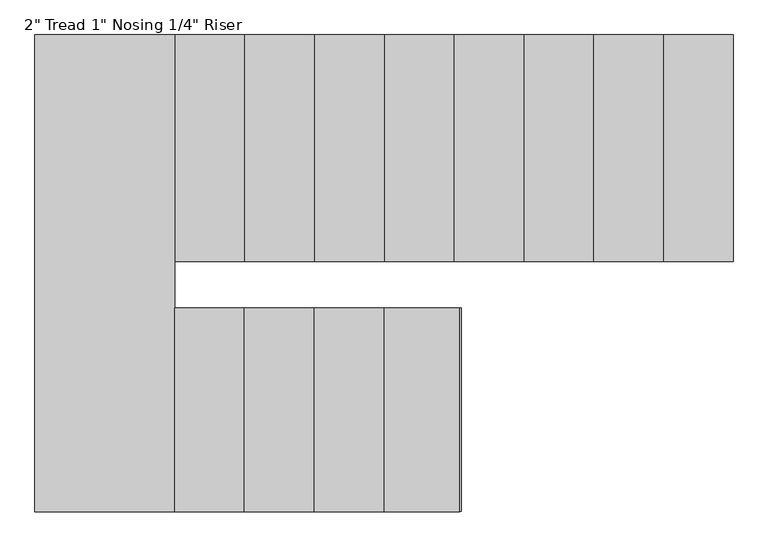
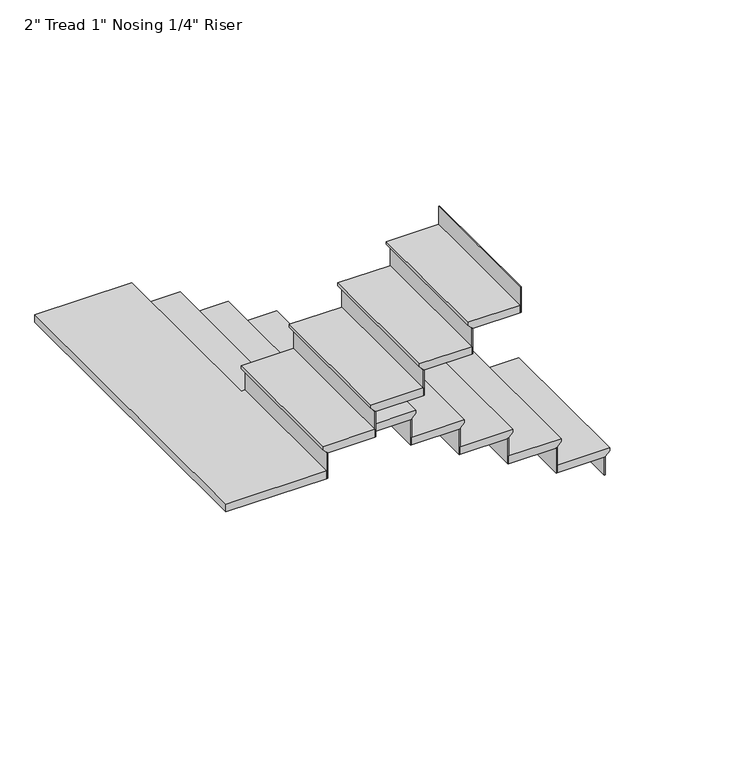
"""IFC4 building model written with IfcOpenShell, lengths in millimetres: stair flight geometry."""

from ifc_helpers import new_model, si_unit, origin, place, context, project, spatial, faceted_brep, source, transform, mapped, element, save


def stair_flight_2d4ab5d3(model_context):
    return source(origin(), model_context, "Body", "Brep", [
        faceted_brep([(-569.5630704, 657.3457979, 12799.4833333), (-569.5630704, 657.3457979, 12818.5333333), (-569.5630704, -333.2542021, 12818.5333333), (-569.5630704, -333.2542021, 12799.4833333), (-594.9630704, 657.3457979, 12774.0833333), (-594.9630704, -333.2542021, 12774.0833333), (-899.7630704, 657.3457979, 12818.5333333), (-899.7630704, -333.2542021, 12818.5333333), (-594.9630704, -333.2542021, 12767.7333333), (-899.7630704, -333.2542021, 12767.7333333), (-899.7630704, 657.3457979, 12767.7333333), (-594.9630704, 657.3457979, 12767.7333333)], [[[0, 1, 2, 3]], [[4, 0, 3, 5]], [[2, 1, 6, 7]], [[8, 9, 10, 11]], [[2, 7, 9, 8, 5, 3]], [[8, 11, 4, 5]], [[6, 1, 0, 4, 11, 10]], [[7, 6, 10, 9]]]),
        faceted_brep([(-594.9630704, 657.3457979, 12767.7333333), (-594.9630704, 657.3457979, 12649.2), (-601.3130704, 657.3457979, 12649.2), (-601.3130704, 657.3457979, 12767.7333333), (-594.9630704, -333.2542021, 12767.7333333), (-601.3130704, -333.2542021, 12767.7333333), (-601.3130704, -333.2542021, 12649.2), (-594.9630704, -333.2542021, 12649.2)], [[[0, 1, 2, 3]], [[4, 5, 6, 7]], [[1, 0, 4, 7]], [[2, 1, 7, 6]], [[3, 2, 6, 5]], [[0, 3, 5, 4]]]),
        faceted_brep([(-899.7630704, 657.3457979, 12937.0666667), (-899.7630704, 657.3457979, 12767.7333333), (-906.1130704, 657.3457979, 12767.7333333), (-906.1130704, 657.3457979, 12937.0666667), (-899.7630704, -333.2542021, 12937.0666667), (-906.1130704, -333.2542021, 12937.0666667), (-906.1130704, -333.2542021, 12767.7333333), (-899.7630704, -333.2542021, 12767.7333333)], [[[0, 1, 2, 3]], [[4, 5, 6, 7]], [[1, 0, 4, 7]], [[2, 1, 7, 6]], [[3, 2, 6, 5]], [[0, 3, 5, 4]]]),
        faceted_brep([(-874.3630704, -333.2542021, 12987.8666667), (-874.3630704, 657.3457979, 12987.8666667), (-1204.5630704, 657.3457979, 12987.8666667), (-1204.5630704, -333.2542021, 12987.8666667), (-899.7630704, -333.2542021, 12937.0666667), (-1204.5630704, -333.2542021, 12937.0666667), (-1204.5630704, 657.3457979, 12937.0666667), (-899.7630704, 657.3457979, 12937.0666667), (-899.7630704, -333.2542021, 12943.4166667), (-874.3630704, -333.2542021, 12968.8166667), (-899.7630704, 657.3457979, 12943.4166667), (-874.3630704, 657.3457979, 12968.8166667)], [[[0, 1, 2, 3]], [[4, 5, 6, 7]], [[0, 3, 5, 4, 8, 9]], [[4, 7, 10, 8]], [[2, 1, 11, 10, 7, 6]], [[3, 2, 6, 5]], [[11, 1, 0, 9]], [[10, 11, 9, 8]]]),
        faceted_brep([(-1204.5630704, 657.3457979, 13106.4), (-1204.5630704, 657.3457979, 12937.0666667), (-1210.9130704, 657.3457979, 12937.0666667), (-1210.9130704, 657.3457979, 13106.4), (-1204.5630704, -333.2542021, 13106.4), (-1210.9130704, -333.2542021, 13106.4), (-1210.9130704, -333.2542021, 12937.0666667), (-1204.5630704, -333.2542021, 12937.0666667)], [[[0, 1, 2, 3]], [[4, 5, 6, 7]], [[1, 0, 4, 7]], [[2, 1, 7, 6]], [[3, 2, 6, 5]], [[0, 3, 5, 4]]]),
        faceted_brep([(-1179.1630704, -333.2542021, 13157.2), (-1179.1630704, 657.3457979, 13157.2), (-1509.3630704, 657.3457979, 13157.2), (-1509.3630704, -333.2542021, 13157.2), (-1204.5630704, -333.2542021, 13106.4), (-1509.3630704, -333.2542021, 13106.4), (-1509.3630704, 657.3457979, 13106.4), (-1204.5630704, 657.3457979, 13106.4), (-1204.5630704, -333.2542021, 13112.75), (-1179.1630704, -333.2542021, 13138.15), (-1204.5630704, 657.3457979, 13112.75), (-1179.1630704, 657.3457979, 13138.15)], [[[0, 1, 2, 3]], [[4, 5, 6, 7]], [[0, 3, 5, 4, 8, 9]], [[4, 7, 10, 8]], [[2, 1, 11, 10, 7, 6]], [[3, 2, 6, 5]], [[11, 1, 0, 9]], [[10, 11, 9, 8]]]),
        faceted_brep([(-1509.3630704, 657.3457979, 13275.7333333), (-1509.3630704, 657.3457979, 13106.4), (-1515.7130704, 657.3457979, 13106.4), (-1515.7130704, 657.3457979, 13275.7333333), (-1509.3630704, -333.2542021, 13275.7333333), (-1515.7130704, -333.2542021, 13275.7333333), (-1515.7130704, -333.2542021, 13106.4), (-1509.3630704, -333.2542021, 13106.4)], [[[0, 1, 2, 3]], [[4, 5, 6, 7]], [[1, 0, 4, 7]], [[2, 1, 7, 6]], [[3, 2, 6, 5]], [[0, 3, 5, 4]]]),
        faceted_brep([(-1483.9630704, -333.2542021, 13326.5333333), (-1483.9630704, 657.3457979, 13326.5333333), (-1814.1630704, 657.3457979, 13326.5333333), (-1814.1630704, -333.2542021, 13326.5333333), (-1509.3630704, -333.2542021, 13275.7333333), (-1814.1630704, -333.2542021, 13275.7333333), (-1814.1630704, 657.3457979, 13275.7333333), (-1509.3630704, 657.3457979, 13275.7333333), (-1509.3630704, -333.2542021, 13282.0833333), (-1483.9630704, -333.2542021, 13307.4833333), (-1509.3630704, 657.3457979, 13282.0833333), (-1483.9630704, 657.3457979, 13307.4833333)], [[[0, 1, 2, 3]], [[4, 5, 6, 7]], [[0, 3, 5, 4, 8, 9]], [[4, 7, 10, 8]], [[2, 1, 11, 10, 7, 6]], [[3, 2, 6, 5]], [[11, 1, 0, 9]], [[10, 11, 9, 8]]]),
        faceted_brep([(-1814.1630704, 657.3457979, 13445.0666667), (-1814.1630704, 657.3457979, 13275.7333333), (-1820.5130704, 657.3457979, 13275.7333333), (-1820.5130704, 657.3457979, 13445.0666667), (-1814.1630704, -333.2542021, 13445.0666667), (-1820.5130704, -333.2542021, 13445.0666667), (-1820.5130704, -333.2542021, 13275.7333333), (-1814.1630704, -333.2542021, 13275.7333333)], [[[0, 1, 2, 3]], [[4, 5, 6, 7]], [[1, 0, 4, 7]], [[2, 1, 7, 6]], [[3, 2, 6, 5]], [[0, 3, 5, 4]]]),
        faceted_brep([(-1788.7630704, -333.2542021, 13495.8666667), (-1788.7630704, 657.3457979, 13495.8666667), (-2118.9630704, 657.3457979, 13495.8666667), (-2118.9630704, -333.2542021, 13495.8666667), (-1814.1630704, -333.2542021, 13445.0666667), (-2118.9630704, -333.2542021, 13445.0666667), (-2118.9630704, 657.3457979, 13445.0666667), (-1814.1630704, 657.3457979, 13445.0666667), (-1814.1630704, -333.2542021, 13451.4166667), (-1788.7630704, -333.2542021, 13476.8166667), (-1814.1630704, 657.3457979, 13451.4166667), (-1788.7630704, 657.3457979, 13476.8166667)], [[[0, 1, 2, 3]], [[4, 5, 6, 7]], [[0, 3, 5, 4, 8, 9]], [[4, 7, 10, 8]], [[2, 1, 11, 10, 7, 6]], [[3, 2, 6, 5]], [[11, 1, 0, 9]], [[10, 11, 9, 8]]]),
        faceted_brep([(-2118.9630704, 657.3457979, 13614.4), (-2118.9630704, 657.3457979, 13445.0666667), (-2125.3130704, 657.3457979, 13445.0666667), (-2125.3130704, 657.3457979, 13614.4), (-2118.9630704, -333.2542021, 13614.4), (-2125.3130704, -333.2542021, 13614.4), (-2125.3130704, -333.2542021, 13445.0666667), (-2118.9630704, -333.2542021, 13445.0666667)], [[[0, 1, 2, 3]], [[4, 5, 6, 7]], [[1, 0, 4, 7]], [[2, 1, 7, 6]], [[3, 2, 6, 5]], [[0, 3, 5, 4]]]),
        faceted_brep([(-2093.5630704, -333.2542021, 13665.2), (-2093.5630704, 657.3457979, 13665.2), (-2423.7630704, 657.3457979, 13665.2), (-2423.7630704, -333.2542021, 13665.2), (-2118.9630704, -333.2542021, 13614.4), (-2423.7630704, -333.2542021, 13614.4), (-2423.7630704, 657.3457979, 13614.4), (-2118.9630704, 657.3457979, 13614.4), (-2118.9630704, -333.2542021, 13620.75), (-2093.5630704, -333.2542021, 13646.15), (-2118.9630704, 657.3457979, 13620.75), (-2093.5630704, 657.3457979, 13646.15)], [[[0, 1, 2, 3]], [[4, 5, 6, 7]], [[0, 3, 5, 4, 8, 9]], [[4, 7, 10, 8]], [[2, 1, 11, 10, 7, 6]], [[3, 2, 6, 5]], [[11, 1, 0, 9]], [[10, 11, 9, 8]]]),
        faceted_brep([(-2423.7630704, 657.3457979, 13783.7333333), (-2423.7630704, 657.3457979, 13614.4), (-2430.1130704, 657.3457979, 13614.4), (-2430.1130704, 657.3457979, 13783.7333333), (-2423.7630704, -333.2542021, 13783.7333333), (-2430.1130704, -333.2542021, 13783.7333333), (-2430.1130704, -333.2542021, 13614.4), (-2423.7630704, -333.2542021, 13614.4)], [[[0, 1, 2, 3]], [[4, 5, 6, 7]], [[1, 0, 4, 7]], [[2, 1, 7, 6]], [[3, 2, 6, 5]], [[0, 3, 5, 4]]]),
        faceted_brep([(-2398.3630704, -333.2542021, 13834.5333333), (-2398.3630704, 657.3457979, 13834.5333333), (-2728.5630704, 657.3457979, 13834.5333333), (-2728.5630704, -333.2542021, 13834.5333333), (-2423.7630704, -333.2542021, 13783.7333333), (-2728.5630704, -333.2542021, 13783.7333333), (-2728.5630704, 657.3457979, 13783.7333333), (-2423.7630704, 657.3457979, 13783.7333333), (-2423.7630704, -333.2542021, 13790.0833333), (-2398.3630704, -333.2542021, 13815.4833333), (-2423.7630704, 657.3457979, 13790.0833333), (-2398.3630704, 657.3457979, 13815.4833333)], [[[0, 1, 2, 3]], [[4, 5, 6, 7]], [[0, 3, 5, 4, 8, 9]], [[4, 7, 10, 8]], [[2, 1, 11, 10, 7, 6]], [[3, 2, 6, 5]], [[11, 1, 0, 9]], [[10, 11, 9, 8]]]),
        faceted_brep([(-2728.5630704, 657.3457979, 13953.0666667), (-2728.5630704, 657.3457979, 13783.7333333), (-2734.9130704, 657.3457979, 13783.7333333), (-2734.9130704, 657.3457979, 13953.0666667), (-2728.5630704, -333.2542021, 13953.0666667), (-2734.9130704, -333.2542021, 13953.0666667), (-2734.9130704, -333.2542021, 13783.7333333), (-2728.5630704, -333.2542021, 13783.7333333)], [[[0, 1, 2, 3]], [[4, 5, 6, 7]], [[1, 0, 4, 7]], [[2, 1, 7, 6]], [[3, 2, 6, 5]], [[0, 3, 5, 4]]]),
        faceted_brep([(-2703.1630704, -333.2542021, 14003.8666667), (-2703.1630704, 657.3457979, 14003.8666667), (-3033.3630704, 657.3457979, 14003.8666667), (-3033.3630704, -333.2542021, 14003.8666667), (-2728.5630704, -333.2542021, 13953.0666667), (-3033.3630704, -333.2542021, 13953.0666667), (-3033.3630704, 657.3457979, 13953.0666667), (-2728.5630704, 657.3457979, 13953.0666667), (-2728.5630704, -333.2542021, 13959.4166667), (-2703.1630704, -333.2542021, 13984.8166667), (-2728.5630704, 657.3457979, 13959.4166667), (-2703.1630704, 657.3457979, 13984.8166667)], [[[0, 1, 2, 3]], [[4, 5, 6, 7]], [[0, 3, 5, 4, 8, 9]], [[4, 7, 10, 8]], [[2, 1, 11, 10, 7, 6]], [[3, 2, 6, 5]], [[11, 1, 0, 9]], [[10, 11, 9, 8]]]),
        faceted_brep([(-3033.3630704, 657.3457979, 14122.4), (-3033.3630704, 657.3457979, 13953.0666667), (-3039.7130704, 657.3457979, 13953.0666667), (-3039.7130704, 657.3457979, 14122.4), (-3033.3630704, -333.2542021, 14122.4), (-3039.7130704, -333.2542021, 14122.4), (-3039.7130704, -333.2542021, 13953.0666667), (-3033.3630704, -333.2542021, 13953.0666667)], [[[0, 1, 2, 3]], [[4, 5, 6, 7]], [[1, 0, 4, 7]], [[2, 1, 7, 6]], [[3, 2, 6, 5]], [[0, 3, 5, 4]]]),
        faceted_brep([(-2982.5630704, -536.4542021, 14173.2), (-3007.9630704, -536.4542021, 14173.2), (-3007.9630704, 657.3457979, 14173.2), (-3617.5630704, 657.3457979, 14173.2), (-3617.5630704, -1425.4542021, 14173.2), (-2982.5630704, -1425.4542021, 14173.2), (-3007.9630704, -536.4542021, 14122.4), (-2982.5630704, -536.4542021, 14122.4), (-2982.5630704, -1425.4542021, 14122.4), (-3617.5630704, -1425.4542021, 14122.4), (-3617.5630704, 657.3457979, 14122.4), (-3033.3630704, 657.3457979, 14122.4), (-3033.3630704, -333.2542021, 14122.4), (-3007.9630704, -333.2542021, 14122.4), (-3007.9630704, -333.2542021, 14154.15), (-3007.9630704, 657.3457979, 14154.15), (-3033.3630704, -333.2542021, 14128.75), (-3033.3630704, 657.3457979, 14128.75)], [[[0, 1, 2, 3, 4, 5]], [[6, 7, 8, 9, 10, 11, 12, 13]], [[1, 0, 7, 6]], [[2, 1, 6, 13, 14, 15]], [[13, 12, 16, 14]], [[12, 11, 17, 16]], [[3, 2, 15, 17, 11, 10]], [[4, 3, 10, 9]], [[5, 4, 9, 8]], [[0, 5, 8, 7]], [[17, 15, 14, 16]]]),
        faceted_brep([(-2982.5630704, -1425.4542021, 14291.7333333), (-2982.5630704, -1425.4542021, 14122.4), (-2976.2130704, -1425.4542021, 14122.4), (-2976.2130704, -1425.4542021, 14291.7333333), (-2982.5630704, -536.4542021, 14291.7333333), (-2976.2130704, -536.4542021, 14291.7333333), (-2976.2130704, -536.4542021, 14122.4), (-2982.5630704, -536.4542021, 14122.4)], [[[0, 1, 2, 3]], [[4, 5, 6, 7]], [[1, 0, 4, 7]], [[2, 1, 7, 6]], [[3, 2, 6, 5]], [[0, 3, 5, 4]]]),
        faceted_brep([(-3007.9630704, -536.4542021, 14342.5333333), (-3007.9630704, -1425.4542021, 14342.5333333), (-2677.7630704, -1425.4542021, 14342.5333333), (-2677.7630704, -536.4542021, 14342.5333333), (-2982.5630704, -536.4542021, 14291.7333333), (-2677.7630704, -536.4542021, 14291.7333333), (-2677.7630704, -1425.4542021, 14291.7333333), (-2982.5630704, -1425.4542021, 14291.7333333), (-2982.5630704, -536.4542021, 14298.0833333), (-3007.9630704, -536.4542021, 14323.4833333), (-2982.5630704, -1425.4542021, 14298.0833333), (-3007.9630704, -1425.4542021, 14323.4833333)], [[[0, 1, 2, 3]], [[4, 5, 6, 7]], [[0, 3, 5, 4, 8, 9]], [[4, 7, 10, 8]], [[2, 1, 11, 10, 7, 6]], [[3, 2, 6, 5]], [[11, 1, 0, 9]], [[10, 11, 9, 8]]]),
        faceted_brep([(-2677.7630704, -1425.4542021, 14461.0666667), (-2677.7630704, -1425.4542021, 14291.7333333), (-2671.4130704, -1425.4542021, 14291.7333333), (-2671.4130704, -1425.4542021, 14461.0666667), (-2677.7630704, -536.4542021, 14461.0666667), (-2671.4130704, -536.4542021, 14461.0666667), (-2671.4130704, -536.4542021, 14291.7333333), (-2677.7630704, -536.4542021, 14291.7333333)], [[[0, 1, 2, 3]], [[4, 5, 6, 7]], [[1, 0, 4, 7]], [[2, 1, 7, 6]], [[3, 2, 6, 5]], [[0, 3, 5, 4]]]),
        faceted_brep([(-2703.1630704, -536.4542021, 14511.8666667), (-2703.1630704, -1425.4542021, 14511.8666667), (-2372.9630704, -1425.4542021, 14511.8666667), (-2372.9630704, -536.4542021, 14511.8666667), (-2677.7630704, -536.4542021, 14461.0666667), (-2372.9630704, -536.4542021, 14461.0666667), (-2372.9630704, -1425.4542021, 14461.0666667), (-2677.7630704, -1425.4542021, 14461.0666667), (-2677.7630704, -536.4542021, 14467.4166667), (-2703.1630704, -536.4542021, 14492.8166667), (-2677.7630704, -1425.4542021, 14467.4166667), (-2703.1630704, -1425.4542021, 14492.8166667)], [[[0, 1, 2, 3]], [[4, 5, 6, 7]], [[0, 3, 5, 4, 8, 9]], [[4, 7, 10, 8]], [[2, 1, 11, 10, 7, 6]], [[3, 2, 6, 5]], [[11, 1, 0, 9]], [[10, 11, 9, 8]]]),
        faceted_brep([(-2372.9630704, -1425.4542021, 14630.4), (-2372.9630704, -1425.4542021, 14461.0666667), (-2366.6130704, -1425.4542021, 14461.0666667), (-2366.6130704, -1425.4542021, 14630.4), (-2372.9630704, -536.4542021, 14630.4), (-2366.6130704, -536.4542021, 14630.4), (-2366.6130704, -536.4542021, 14461.0666667), (-2372.9630704, -536.4542021, 14461.0666667)], [[[0, 1, 2, 3]], [[4, 5, 6, 7]], [[1, 0, 4, 7]], [[2, 1, 7, 6]], [[3, 2, 6, 5]], [[0, 3, 5, 4]]]),
        faceted_brep([(-2398.3630704, -536.4542021, 14681.2), (-2398.3630704, -1425.4542021, 14681.2), (-2068.1630704, -1425.4542021, 14681.2), (-2068.1630704, -536.4542021, 14681.2), (-2372.9630704, -536.4542021, 14630.4), (-2068.1630704, -536.4542021, 14630.4), (-2068.1630704, -1425.4542021, 14630.4), (-2372.9630704, -1425.4542021, 14630.4), (-2372.9630704, -536.4542021, 14636.75), (-2398.3630704, -536.4542021, 14662.15), (-2372.9630704, -1425.4542021, 14636.75), (-2398.3630704, -1425.4542021, 14662.15)], [[[0, 1, 2, 3]], [[4, 5, 6, 7]], [[0, 3, 5, 4, 8, 9]], [[4, 7, 10, 8]], [[2, 1, 11, 10, 7, 6]], [[3, 2, 6, 5]], [[11, 1, 0, 9]], [[10, 11, 9, 8]]]),
        faceted_brep([(-2068.1630704, -1425.4542021, 14799.7333333), (-2068.1630704, -1425.4542021, 14630.4), (-2061.8130704, -1425.4542021, 14630.4), (-2061.8130704, -1425.4542021, 14799.7333333), (-2068.1630704, -536.4542021, 14799.7333333), (-2061.8130704, -536.4542021, 14799.7333333), (-2061.8130704, -536.4542021, 14630.4), (-2068.1630704, -536.4542021, 14630.4)], [[[0, 1, 2, 3]], [[4, 5, 6, 7]], [[1, 0, 4, 7]], [[2, 1, 7, 6]], [[3, 2, 6, 5]], [[0, 3, 5, 4]]]),
        faceted_brep([(-1763.3630704, -1425.4542021, 14969.0666667), (-1763.3630704, -1425.4542021, 14799.7333333), (-1757.0130704, -1425.4542021, 14799.7333333), (-1757.0130704, -1425.4542021, 14969.0666667), (-1763.3630704, -536.4542021, 14969.0666667), (-1757.0130704, -536.4542021, 14969.0666667), (-1757.0130704, -536.4542021, 14799.7333333), (-1763.3630704, -536.4542021, 14799.7333333)], [[[0, 1, 2, 3]], [[4, 5, 6, 7]], [[1, 0, 4, 7]], [[2, 1, 7, 6]], [[3, 2, 6, 5]], [[0, 3, 5, 4]]]),
        faceted_brep([(-2093.5630704, -536.4542021, 14850.5333333), (-2093.5630704, -1425.4542021, 14850.5333333), (-1763.3630704, -1425.4542021, 14850.5333333), (-1763.3630704, -536.4542021, 14850.5333333), (-2068.1630704, -536.4542021, 14799.7333333), (-1763.3630704, -536.4542021, 14799.7333333), (-1763.3630704, -1425.4542021, 14799.7333333), (-2068.1630704, -1425.4542021, 14799.7333333), (-2068.1630704, -536.4542021, 14806.0833333), (-2093.5630704, -536.4542021, 14831.4833333), (-2068.1630704, -1425.4542021, 14806.0833333), (-2093.5630704, -1425.4542021, 14831.4833333)], [[[0, 1, 2, 3]], [[4, 5, 6, 7]], [[0, 3, 5, 4, 8, 9]], [[4, 7, 10, 8]], [[2, 1, 11, 10, 7, 6]], [[3, 2, 6, 5]], [[11, 1, 0, 9]], [[10, 11, 9, 8]]]),
    ])


if __name__ == "__main__":
    model = new_model("IFC4")
    model_context = context("Model", 3, world=origin())
    ifc_project = project(units=[si_unit("LENGTHUNIT", "METRE", prefix="MILLI")], contexts=[model_context])
    site = spatial("IfcSite", under=ifc_project)
    building = spatial("IfcBuilding", under=site)
    placement = place(None, origin())
    stair_flight_shape = stair_flight_2d4ab5d3(model_context)
    element("IfcStairFlight", 1, ObjectType="2\" Tread 1\" Nosing 1/4\" Riser", at=placement, inside=building, context=model_context, shape_type="MappedRepresentation", body=[
        mapped(stair_flight_shape, transform((0.0, 0.0, 0.0), x_axis=(1.0, 0.0, 0.0), y_axis=(0.0, 1.0, 0.0), z_axis=(0.0, 0.0, 1.0))),
    ])
    save(model, "model.ifc")
